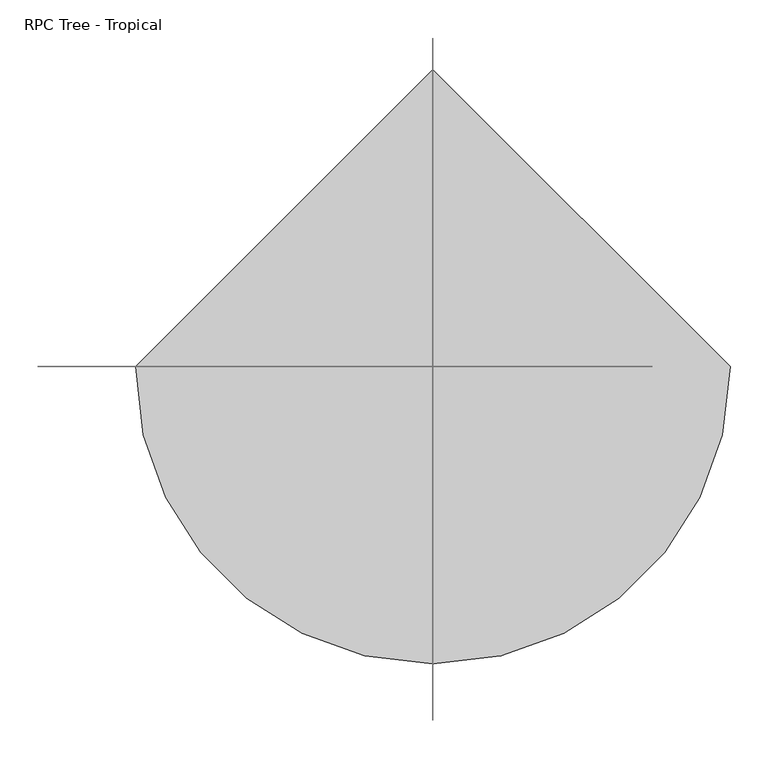
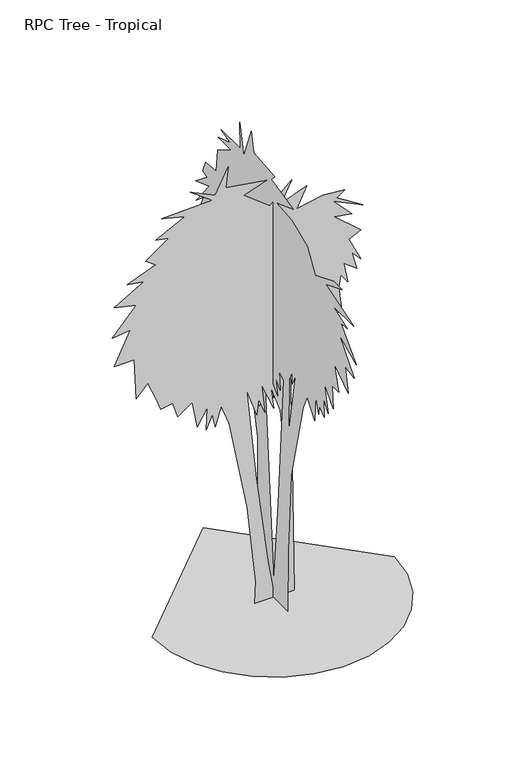
"""IFC4 building model written with IfcOpenShell, lengths in millimetres: geographic element geometry, RPC Tree - Tropical."""

from ifc_helpers import new_model, si_unit, origin, place, context, project, spatial, triangles, source, transform, mapped, element, save


def rpc_tree_tropical_82ff1ee0(model_context):
    return source(origin(), model_context, "Body", "Tessellation", [
        triangles([(0.0, 68.9771396, 618.8468193), (0.0, 81.3218167, 600.9474395), (0.0, 100.5519475, 725.9461687), (0.0, -82.1358931, 0.0), (0.0, -83.3197871, 207.8534466), (0.0, -100.2098081, 479.1084738), (0.0, -168.6723352, 751.584938), (0.0, -191.1077027, 799.6621634), (0.0, -232.7734371, 745.1765356), (0.0, -239.1833838, 834.9174242), (0.0, -255.2095495, 780.4317965), (0.0, -258.4124971, 812.4815844), (0.0, -287.2593374, 790.0457445), (0.0, -284.0538463, 850.9423182), (0.0, -309.6951954, 815.6870573), (0.0, -287.2593374, 905.4280186), (0.0, -335.3340011, 847.7368452), (0.0, -332.1310716, 924.6583855), (0.0, -367.3863324, 924.6583855), (0.0, -342.0142256, 1006.888468), (0.0, -421.8719965, 953.5051712), (0.0, -402.5171459, 1031.9253119), (0.0, -453.9217844, 1024.0157656), (0.0, -371.2242886, 1123.7185461), (0.0, -466.7411691, 1078.5013933), (0.0, -379.5681833, 1169.6164713), (0.0, -416.1264896, 1170.1726873), (0.0, -333.4594789, 1199.982205), (0.0, -450.7162751, 1200.2920698), (0.0, -293.6703014, 1248.3692951), (0.0, -386.6166993, 1286.8300289), (0.0, -338.5395103, 1286.8300289), (0.0, -235.9784014, 1245.1638222), (0.0, -189.6746325, 1315.3974712), (0.0, -104.9042436, 1353.6627228), (0.0, -18.0349252, 1360.5461689), (0.0, -110.9814616, 1395.8014297), (0.0, 10.8103129, 1424.6455994), (0.0, -8.4197106, 1443.8761116), (0.0, 108.6159538, 1455.4355804), (0.0, 122.9870424, 1520.7975792), (0.0, 164.6530312, 1408.6207054), (0.0, 187.0881443, 1511.1836311), (0.0, 183.8834162, 1424.6455994), (0.0, 292.8549624, 1421.4427425), (0.0, 240.050046, 1409.5376553), (0.0, 308.8798745, 1386.1848656), (0.0, 235.1638254, 1386.1848656), (0.0, 312.0853475, 1341.3156567), (0.0, 318.4963297, 1264.3941891), (0.0, 379.3903962, 1257.9832432), (0.0, 395.4152902, 1219.5225094), (0.0, 369.7764845, 1213.1140343), (0.0, 433.8786037, 1161.831336), (0.0, 358.9662068, 1188.3946856), (0.0, 430.6730945, 1097.7317602), (0.0, 389.0068514, 1132.9870211), (0.0, 421.0566393, 1065.6819723), (0.0, 353.7515905, 1126.5760752), (0.0, 417.8511663, 1014.3992741), (0.0, 385.8013784, 1049.6545349), (0.0, 315.2908204, 1120.1676727), (0.0, 382.5958692, 966.3245922), (0.0, 344.1351354, 1011.1963446), (0.0, 353.7515905, 943.8887524), (0.0, 328.1102414, 998.3743801), (0.0, 328.1102414, 918.2473669), (0.0, 315.2908204, 918.2473669), (0.0, 331.3157144, 873.3782307), (0.0, 283.2385072, 889.4031246), (0.0, 324.9047321, 799.6621634), (0.0, 289.6494713, 796.4566904), (0.0, 302.4714176, 713.1242043), (0.0, 280.0355596, 757.9959566), (0.0, 283.2385072, 687.4853622), (0.0, 254.3942104, 745.1765356), (0.0, 244.7792813, 655.435647), (0.0, 231.9590973, 709.9212748), (0.0, 219.1386771, 645.8191555), (0.0, 193.4985997, 671.4604683), (0.0, 174.2682328, 639.4082096), (0.0, 161.4480487, 757.9959566), (0.0, 135.8077261, 645.8191555), (0.0, 132.6024893, 697.0993103), (0.0, 87.4312912, 494.6812151), (0.0, 84.5267992, 0.0), (0.0, 42.8608059, 709.9212748), (0.0, -2.0096292, 684.2798893), (0.0, 20.4257563, 748.3820086), (0.0, -24.4450082, 703.5102562), (0.0, -14.8297941, 757.9959566), (0.0, -40.4701542, 732.3545712), (0.0, -34.0601984, 793.2512175), (0.0, -59.7005347, 777.2263235), (0.0, -26.9908557, 335.1155551), (0.0, -2.0096292, 56.0896632), (0.0, 46.0662925, 693.8938374), (0.0, -107.7764792, 834.9174242), (0.0, -107.7764792, 793.2512175), (0.0, -127.0066009, 838.1229698), (0.0, -87.4922522, 616.758938), (0.0, -88.5461032, 799.6621634), (1.2566193, -3.44e-05, 645.8191555), (-37.2039632, -4.13e-05, 738.7655897), (-27.588773, -3.44e-05, 642.6136826), (-46.8191535, -4.13e-05, 693.8938374), (-53.2293636, -3.44e-05, 642.6136826), (-85.2796511, -4.13e-05, 735.5600441), (-55.1696703, -2.75e-05, 424.8234515), (-17.6170944, -6.9e-06, 132.7480291), (1.1592355, 0.0, 15.9178056), (11.5905001, 0.0, 28.4353578), (19.935561, -6.9e-06, 174.4731985), (38.7117087, -2.75e-05, 468.6360025), (22.0217686, -3.44e-05, 631.3640059), (-8.3588267, -4.13e-05, 722.7406958), (-59.6393193, 0.0, 0.0), (-57.2560346, 0.0, 72.2466348), (-84.3771898, -2.06e-05, 335.1155551), (-142.9707881, -3.44e-05, 642.6136826), (-168.6113833, -4.13e-05, 713.1242043), (-187.8412415, -3.44e-05, 649.0246284), (-197.4566975, -4.13e-05, 693.8938374), (-216.6870644, -3.44e-05, 649.0246284), (-213.4818458, -4.13e-05, 722.7406958), (-245.5323785, -4.13e-05, 668.2549953), (-261.5570181, -4.13e-05, 757.9959566), (-309.6342253, -4.13e-05, 725.9461687), (-325.6591192, -4.81e-05, 777.2263235), (-364.1198894, -4.81e-05, 770.8153776), (-376.9393104, -4.81e-05, 806.0706385), (-405.7861324, -4.81e-05, 873.3782307), (-444.2443591, -4.81e-05, 834.9174242), (-450.655305, -5.5e-05, 969.5300652), (-514.7574243, -5.5e-05, 969.5300652), (-463.474726, -6.19e-05, 1075.2959204), (-521.165863, -6.19e-05, 1068.8849018), (-444.2443591, -6.88e-05, 1155.4229336), (-514.7574243, -6.88e-05, 1171.4478275), (-418.6055534, -6.88e-05, 1225.9334553), (-473.0911812, -7.57e-05, 1235.5474033), (-380.1447833, -7.57e-05, 1270.805135), (-412.1945712, -7.57e-05, 1293.238504), (-338.9001715, -8.25e-05, 1346.9494698), (-380.1447833, -8.25e-05, 1354.1350777), (-287.1983673, -8.25e-05, 1402.2123756), (-360.9144164, -8.25e-05, 1421.4401264), (-197.4566975, -8.25e-05, 1427.8512177), (-267.9680004, -8.94e-05, 1479.1313725), (-187.8412415, -8.25e-05, 1440.6731094), (-146.1757705, -8.94e-05, 1524.0030521), (-153.2237688, -8.25e-05, 1455.4355804), (-21.178765, -8.25e-05, 1434.2621635), (-94.8948436, -8.25e-05, 1408.6207054), (-11.5635259, -8.25e-05, 1344.5212749), (59.5745477, -8.25e-05, 1407.4498466), (23.691668, -7.57e-05, 1338.1101837), (108.2181855, -8.25e-05, 1370.1295956), (76.2893023, -7.57e-05, 1302.3062645), (160.5267932, -7.57e-05, 1319.5021626), (232.0200674, -7.57e-05, 1312.4688709), (205.3192808, -7.57e-05, 1295.4712166), (289.7104414, -7.57e-05, 1241.9583492), (193.5598241, -7.57e-05, 1286.8300289), (253.5961305, -6.88e-05, 1223.860762), (196.7647884, -7.57e-05, 1232.3444012), (283.3020026, -6.88e-05, 1158.6284065), (244.8404876, -6.88e-05, 1139.3980396), (283.3020026, -6.19e-05, 1059.2710264), (254.4551624, -6.19e-05, 1091.3208143), (270.4800563, -6.19e-05, 1030.424168), (228.8153393, -6.19e-05, 1062.4764994), (241.6355052, -5.5e-05, 995.1689072), (219.2001559, -6.19e-05, 1027.2212385), (212.7899367, -5.5e-05, 985.5549591), (222.4051383, -5.5e-05, 902.222473), (183.9443682, -5.5e-05, 895.8140705), (206.37999, -4.81e-05, 844.5313723), (155.099054, -4.81e-05, 857.3533367), (148.6891073, -4.81e-05, 783.6372694), (119.8432845, -4.81e-05, 796.4566904), (103.8178818, -4.81e-05, 770.8153776), (74.972822, -4.81e-05, 809.2761114), (71.7675898, -4.13e-05, 745.1765356), (55.7421917, -4.81e-05, 767.609832), (61.6606531, -2.75e-05, 431.0820448), (68.5626119, 0.0, 0.0), (-392.2986926, 0.0, 0.0), (-381.9278503, -89.8887448, 0.0), (-352.3901547, -172.4373852, 0.0), (-306.0528305, -245.2804135, 0.0), (-245.2804135, -306.0528305, 0.0), (-172.4373852, -352.3901547, 0.0), (-89.8887448, -381.9278503, 0.0), (1.71e-05, -392.2986926, 0.0), (89.8887448, -381.9278503, 0.0), (172.4373852, -352.3901547, 0.0), (245.2804135, -306.0528305, 0.0), (306.0528305, -245.2804135, 0.0), (352.3901547, -172.4373852, 0.0), (381.9278503, -89.8887448, 0.0), (392.2986926, 3.44e-05, 0.0), (-5.14e-05, 392.2986926, 0.0)], [[94, 4, 5], [4, 94, 95], [94, 5, 6], [42, 43, 44], [55, 56, 57], [59, 60, 61], [44, 45, 46], [4, 95, 96], [82, 83, 84], [62, 63, 64], [64, 65, 66], [28, 29, 30], [72, 73, 74], [46, 47, 48], [53, 54, 55], [76, 77, 78], [26, 27, 28], [24, 25, 26], [14, 15, 16], [10, 11, 12], [59, 61, 62], [57, 58, 59], [30, 31, 32], [30, 32, 33], [98, 99, 100], [74, 75, 76], [102, 98, 93], [40, 41, 42], [36, 37, 38], [86, 4, 96], [89, 90, 91], [80, 81, 82], [16, 17, 18], [102, 93, 94], [91, 92, 93], [87, 88, 89], [8, 9, 10], [22, 23, 24], [20, 21, 22], [12, 13, 14], [38, 39, 40], [101, 102, 94], [101, 94, 6], [101, 6, 7], [100, 101, 7], [100, 7, 8], [68, 69, 70], [78, 79, 80], [85, 86, 96], [85, 96, 97], [78, 80, 82], [70, 71, 72], [55, 57, 59], [18, 19, 20], [10, 12, 14], [51, 52, 53], [50, 51, 53], [76, 78, 82], [66, 67, 68], [44, 46, 48], [20, 22, 24], [42, 44, 48], [55, 59, 62], [50, 53, 55], [100, 8, 10], [10, 14, 16], [24, 26, 28], [62, 64, 66], [50, 55, 62], [16, 18, 20], [100, 10, 16], [38, 40, 42], [36, 38, 42], [48, 49, 50], [28, 30, 33], [72, 74, 76], [72, 76, 82], [70, 72, 82], [89, 91, 93], [3, 20, 24], [3, 24, 28], [3, 28, 33], [3, 33, 34], [3, 34, 35], [3, 35, 36], [3, 36, 42], [3, 42, 48], [3, 48, 50], [3, 50, 62], [3, 62, 66], [3, 66, 68], [3, 68, 70], [3, 70, 82], [3, 82, 84], [2, 3, 84], [2, 84, 85], [100, 16, 20], [1, 2, 85], [1, 85, 97], [3, 1, 97], [3, 97, 87], [3, 87, 89], [98, 100, 20], [98, 20, 3], [93, 98, 3], [93, 3, 89], [162, 163, 164], [148, 149, 150], [104, 105, 106], [116, 103, 104], [110, 117, 118], [168, 169, 170], [146, 147, 148], [150, 151, 152], [123, 124, 125], [155, 156, 157], [172, 173, 174], [106, 107, 108], [117, 110, 111], [187, 117, 111], [152, 153, 154], [121, 122, 123], [140, 141, 142], [144, 145, 146], [170, 171, 172], [164, 165, 166], [160, 161, 162], [183, 184, 185], [110, 118, 119], [109, 110, 119], [109, 119, 120], [108, 109, 120], [125, 126, 127], [136, 137, 138], [138, 139, 140], [157, 158, 159], [132, 133, 134], [108, 120, 121], [177, 178, 179], [104, 106, 108], [187, 111, 112], [134, 135, 136], [160, 162, 164], [166, 167, 168], [181, 182, 183], [186, 187, 112], [186, 112, 113], [186, 113, 114], [185, 186, 114], [185, 114, 115], [185, 115, 116], [179, 180, 181], [142, 143, 144], [127, 128, 129], [121, 123, 125], [175, 176, 177], [129, 130, 131], [179, 181, 183], [185, 116, 104], [150, 152, 154], [148, 150, 154], [159, 160, 164], [159, 164, 166], [168, 170, 172], [183, 185, 104], [166, 168, 172], [159, 166, 172], [159, 172, 174], [129, 131, 132], [159, 174, 175], [159, 175, 177], [159, 177, 179], [159, 179, 183], [159, 183, 104], [159, 104, 108], [157, 159, 108], [155, 157, 108], [155, 108, 121], [155, 121, 125], [155, 125, 127], [155, 127, 129], [155, 129, 132], [155, 132, 134], [155, 134, 136], [155, 136, 138], [155, 138, 140], [155, 140, 142], [154, 155, 142], [154, 142, 144], [148, 154, 144], [146, 148, 144], [202, 203, 188], [201, 202, 188], [201, 188, 189], [200, 201, 189], [200, 189, 190], [200, 190, 191], [199, 200, 191], [198, 199, 191], [198, 191, 192], [198, 192, 193], [198, 193, 194], [198, 194, 195], [198, 195, 196], [198, 196, 197]], closed=False),
    ])


if __name__ == "__main__":
    model = new_model("IFC4")
    model_context = context("Model", 3, world=origin())
    ifc_project = project(units=[si_unit("LENGTHUNIT", "METRE", prefix="MILLI")], contexts=[model_context])
    site = spatial("IfcSite", under=ifc_project)
    building = spatial("IfcBuilding", under=site)
    placement = place(None, origin())
    rpc_tree_tropical_shape = rpc_tree_tropical_82ff1ee0(model_context)
    element("IfcGeographicElement", 1, ObjectType="RPC Tree - Tropical", at=placement, inside=building, context=model_context, shape_type="MappedRepresentation", body=[
        mapped(rpc_tree_tropical_shape, transform((0.0, 0.0, 0.0), x_axis=(1.0, 0.0, 0.0), y_axis=(0.0, 1.0, 0.0), z_axis=(0.0, 0.0, 1.0))),
    ])
    save(model, "model.ifc")

# Revit data of these elements
# Type "RPC Tree - Tropical"
#   built-in parameter 1005198 = "{2, 15},{39, RPC-16-FXGL-GN00-PMD1-0000-ST1L-LVER-AU},{1, 0},{1, 0},{2, 13},{1, 8},{5, Color},{1, 0},{1, 0},{3, 0.8},{3, 0.8},{3, 0.8},{1, 8},{7, BBoxMin},{1, 0},{1, 0},{1, 0},{1, 0},{1, 0},{1, 8},{7, BBoxMax},{1, 0},{1, 0},{1, 0},{1, 0},{1, 0},{2, 11},{9, RPCTypeId},{1, 0},{1, 0},{39, RPC-16-FXGL-GN00-PMD1-0000-ST1L-LVER-AU},{1, 6},{14, RPCPlantHeight},{1, 0},{1, 0},{1, 5},{2, 11},{7, keyword},{1, 0},{1, 0},{35, :RPCs:Trees [Tropical]:Geometry:RPC},{2, 11},{8, category},{1, 0},{1, 0},{16, Trees [Tropical]},{2, 11},{12, LocalizedUID},{1, 0},{1, 0},{19, Buddha Belly Bamboo},{2, 14},{6, Height},{1, 0},{1, 0},{1, 5},{1, 2},{16, Cast Reflections},{1, 0},{1, 0},{1, 0},{1, 2},{12, Cast Shadows},{1, 0},{1, 0},{1, 1},{1, 2},{9, Lock View},{1, 0},{1, 0},{1, 0},{1, 4},{5, ViewC},{1, 0},{1, 0},{1, 0},{21, assetlibrary_base.fbx},{1, 5},"
#   built-in parameter 1005195 = "RPC-16-FXGL-GN00-PMD1-0000-ST1L-LVER-AU"
#   Assembly Code = "G2050500"
#   Height = 5' - 0"
#   Plan Symbol = element 361270
#   Default Elevation = 0
